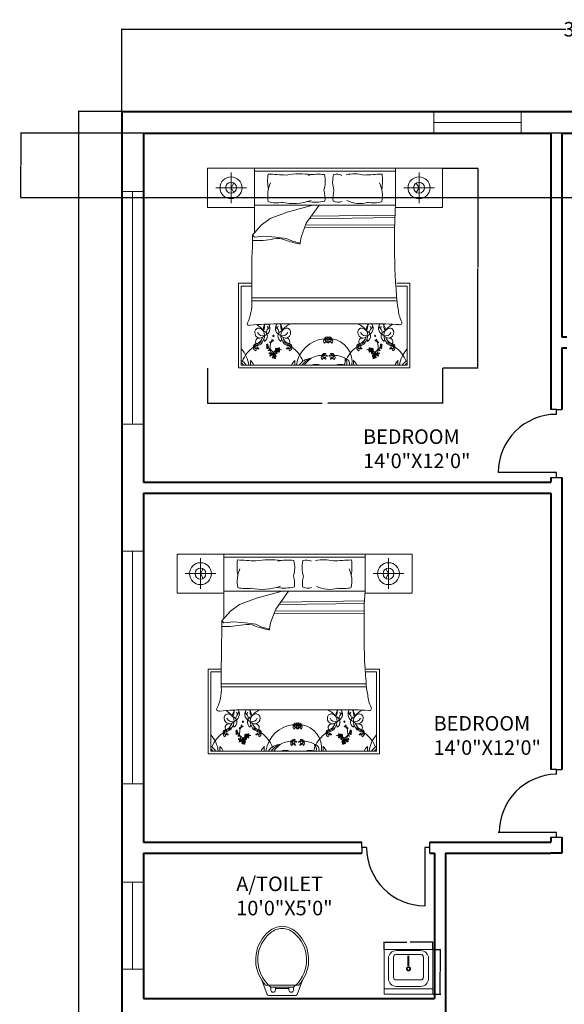
# Model space of a CAD drawing. Units: inches. Extents: x -19 to 419, y -828 to 43.
# Tile 8 of 9: x -19 to 205, y -364 to 43. Entities that reach past the tile are written whole.
import ezdxf

# ---------------------------------------------------------------- set-up
doc = ezdxf.new("R2010")
doc.units = ezdxf.units.IN
doc.header["$MEASUREMENT"] = 0
for name, color, linetype, lineweight in [('A-ANNO-DIMS', 2, 'Continuous', 18), ('A-AREA-IDEN', 7, 'Continuous', 25), ('A-DOOR', 3, 'Continuous', 25), ('A-FLOR-FIXT', 9, 'Continuous', 20), ('A-FURN', 8, 'Continuous', 18), ('A-GLAZ', 4, 'Continuous', 20), ('A-WALL', 7, 'Continuous', 40)]:
    doc.layers.add(name, color=color, linetype=linetype, lineweight=lineweight)
doc.styles.get("Standard").update_dxf_attribs({"font": 'arial.ttf'})
doc.dimstyles.get("Standard").update_dxf_attribs({"dimtxt": 0.18, "dimasz": 0.18, "dimexe": 0.18, "dimexo": 0.0625, "dimgap": 0.09, "dimtad": 0, "dimtih": 1, "dimtoh": 1, "dimdec": 0, "dimzin": 0, "dimdsep": 46, "dimlunit": 3, "dimtxsty": 'Standard', "dimcen": 0.09, "dimadec": 0, "dimazin": 0, "dimtfac": 1, "dimtdec": 0, "dimtofl": 0, "dimtmove": 0, "dimatfit": 3, "dimfxl": 1, "dimtolj": 1, "dimtzin": 0, "dimarcsym": 0})

# ---------------------------------------------------------------- blocks, each defined once
blk = doc.blocks.new('*D1')
at = {"layer": 'A-ANNO-DIMS', "color": 0, "lineweight": -2, "transparency": 16777216}
for p, q in [((22.74, 4.83), (22.74, 38.87)), ((22.92, 38.69), (205.85, 38.69)), ((409.56, 38.69), (226.63, 38.69)), ((409.74, 4.83), (409.74, 38.87))]:
    blk.add_line(p, q, dxfattribs=at)
at = {"layer": 'A-ANNO-DIMS', "color": 0, "transparency": 16777216}
for points in [[(22.92, 38.72), (22.92, 38.66), (22.74, 38.69)], [(409.56, 38.72), (409.56, 38.66), (409.74, 38.69)]]:
    blk.add_solid(points, dxfattribs=at)
at = {"layer": 'Defpoints', "color": 0, "transparency": 16777216}
for p in [(409.74, 38.69), (22.74, 4.77), (409.74, 4.77)]:
    blk.add_point(p, dxfattribs=at)
at = {"layer": 'A-ANNO-DIMS', "color": 0, "transparency": 16777216, "insert": (216.24, 38.69), "char_height": 6, "attachment_point": 5}
blk.add_mtext('\\A1;32\'-3"', dxfattribs=at)
blk = doc.blocks.new('*D2')
at = {"layer": 'A-ANNO-DIMS', "color": 0, "lineweight": -2, "transparency": 16777216}
for p, q in [((22.68, 4.77), (4.74, 4.77)), ((4.92, 4.59), (4.92, -387.33)), ((4.92, -785.55), (4.92, -393.64)), ((22.68, -785.73), (4.74, -785.73))]:
    blk.add_line(p, q, dxfattribs=at)
at = {"layer": 'A-ANNO-DIMS', "color": 0, "transparency": 16777216}
for points in [[(4.89, 4.59), (4.95, 4.59), (4.92, 4.77)], [(4.89, -785.55), (4.95, -785.55), (4.92, -785.73)]]:
    blk.add_solid(points, dxfattribs=at)
at = {"layer": 'Defpoints', "color": 0, "transparency": 16777216}
for p in [(22.74, 4.77), (4.92, -785.73), (22.74, -785.73)]:
    blk.add_point(p, dxfattribs=at)
at = {"layer": 'A-ANNO-DIMS', "color": 0, "transparency": 16777216, "insert": (4.92, -390.48), "char_height": 6, "attachment_point": 5}
blk.add_mtext('\\A1;65\'-11"', dxfattribs=at)
blk = doc.blocks.new('М14 600х655')
for p, q in [((-655, 600), (-655, 0)), ((-655, 600), (-655, 0)), ((-655, 0), (-655, 600)), ((0, 600), (-655, 600)), ((0, 0), (0, 600)), ((0, 525), (-655, 525)), ((-165, 494), (-490, 494)), ((-165, 408), (-490, 408)), ((-596, 388), (-596, 121)), ((-528, 370), (-528, 103)), ((-127, 103), (-127, 370)), ((-59, 121), (-59, 388)), ((-334, 87), (-334, 220)), ((-321, 87), (-321, 220)), ((-655, 0), (-655, 0)), ((-655, 0), (-655, 0)), ((-655, 0), (0, 0)), ((-655, 0), (0, 0)), ((-490, 65), (-165, 65)), ((-490, 15), (-165, 15))]:
    blk.add_line(p, q)
for radius in [27.6, 19.3]:
    blk.add_circle((-327, 259), radius)
for centre, radius, start, end in [((-490, 388), 106, 90, 180), ((-490, 370), 38.2, 90, 180), ((-165, 388), 106, 0, 90), ((-165, 370), 38.2, 0, 90), ((-490, 121), 106, 180, 270), ((-490, 103), 38.2, 180, 270), ((-165, 121), 106, 270, 0), ((-165, 103), 38.2, 270, 0)]:
    blk.add_arc(centre, radius, start, end)
blk = doc.blocks.new('WIN-36X9')
for p, q in [((36, 9), (0, 9)), ((0, 9), (0, 0)), ((36, 0), (36, 9)), ((0, 4.5), (36, 4.5)), ((0, 0), (36, 0))]:
    blk.add_line(p, q)
blk = doc.blocks.new('WIN-96X9')
for p, q in [((96, 9), (0, 9)), ((0, 9), (0, 0)), ((96, 0), (96, 9)), ((0, 4.5), (96, 4.5)), ((0, 0), (96, 0))]:
    blk.add_line(p, q)
blk = doc.blocks.new('DOOR-24-PARTITION')
for p, q in [((2, 2.25), (2, 26.25)), ((0, 4.5), (0, 0)), ((28, 2.25), (28, 4.5)), ((0, 2.25), (2, 2.25)), ((26, 2.25), (28, 2.25)), ((28, 2.25), (28, 0))]:
    blk.add_line(p, q)
blk.add_arc((2, 2.25), 24, 0, 90)
blk = doc.blocks.new('BED-DOUBLE-WITH-NIGHTSTANDS')
for p, q in [((0, 82.42), (96.91, 82.42)), ((19.38, 82.42), (19.38, 55.82)), ((9.69, 68.01), (9.69, 80.67)), ((77.53, 81.17), (19.38, 81.17)), ((87.22, 68.01), (87.22, 80.67)), ((16.02, 74.34), (3.36, 74.34)), ((80.89, 74.34), (93.55, 74.34)), ((19.38, 67.1), (77.53, 67.1)), ((32.84, 64.22), (43.41, 67.1)), ((46.01, 67.1), (40.69, 59.71)), ((22.05, 58.92), (25.78, 61.67)), ((25.78, 61.67), (32.84, 64.22)), ((77.23, 62.08), (42.04, 61.58)), ((77.27, 63.07), (42.77, 62.59)), ((18.51, 54.8), (22.05, 58.92)), ((40.69, 59.71), (38.54, 54.02)), ((77.19, 58.03), (40, 57.88)), ((77.18, 59.03), (40.38, 58.88)), ((19.3, 54.02), (18.51, 54.8)), ((23.23, 54.41), (19.3, 54.02)), ((28.13, 54.02), (23.23, 54.41)), ((32.45, 53.43), (28.13, 54.02)), ((35, 52.25), (32.45, 53.43)), ((38.54, 54.02), (38.14, 51.47)), ((38.14, 51.47), (35, 52.25)), ((12.79, 34.91), (18.27, 34.91)), ((12.79, 0), (12.79, 34.91)), ((18.27, 33.79), (13.91, 33.79)), ((13.91, 33.79), (13.91, 1.12)), ((82.32, 33.79), (78.05, 33.79)), ((78.07, 34.91), (83.44, 34.91)), ((82.32, 1.12), (82.32, 33.79)), ((83.44, 34.91), (83.44, 0)), ((77.97, 28.87), (18.27, 28.87)), ((78.06, 27.66), (18.27, 27.66)), ((68.13, 18.14), (28.78, 18.14)), ((23.46, 10.95), (23.25, 12.04)), ((30.24, 10.95), (30.45, 12.04)), ((66, 10.95), (65.78, 12.04)), ((72.77, 10.95), (72.98, 12.04)), ((13.91, 1.12), (82.32, 1.12)), ((83.44, 0), (12.79, 0))]:
    blk.add_line(p, q)
for points in [[(19.38, 66.26), (0, 66.26), (0, 82.42)], [(77.53, 82.42), (77.53, 66.26), (96.91, 66.26), (96.91, 82.42)], [(9.69, 74.34), (10.82, 76.3)], [(9.69, 74.34), (10.82, 72.38)], [(87.22, 74.34), (86.09, 76.3)], [(87.22, 74.34), (86.09, 72.38)]]:
    blk.add_lwpolyline(points)
for points in [[(24.95, 80, 0.074897), (25.07, 73.67, -0.472817)], [(48, 73.32, 0.14099), (48.19, 79.77, 0.235245)], [(52.14, 73.32, -0.14099), (51.95, 79.77, -0.235245)], [(71.96, 80, -0.074897), (71.84, 73.67, 0.472817)], [(18.31, 45.93, 0.001242), (18.27, 27.54, -0.127202), (16.32, 18.38)], [(77.94, 29.63, 0.056112), (78.64, 24.3, 0.095341), (80.01, 19.16)]]:
    blk.add_lwpolyline(points, format="xyb")
for centre, radius in [((9.69, 74.34), 4.52), ((87.22, 74.34), 4.52), ((9.69, 74.34), 2.26), ((87.22, 74.34), 2.26), ((27.45, 4.83), 0.247), ((29.06, 7.44), 0.247), ((67.17, 7.44), 0.247), ((68.79, 4.83), 0.247)]:
    blk.add_circle(centre, radius)
for centre, radius, start, end in [((78.36, 1002.26), 923.81, 266.68521, 267.14978), ((38.23, 44.93), 35.15, 82.2196, 99.497), ((45.65, 62.69), 17.27, 81.5249, 103.96), ((53.28, 75.17), 4.79, 63.3437, 106.1026), ((60.46, 63.04), 17.04, 76.3427, 101.1841), ((18.55, 1002.26), 923.81, 272.85022, 273.31479), ((37.29, 71.13), 12.49, 155.1316, 191.7583), ((36.58, 70.08), 11.87, 354.0129, 15.8293), ((63.56, 70.08), 11.87, 164.1707, 185.9871), ((59.62, 71.13), 12.49, 348.2417, 24.8684), ((35.24, 90.37), 22.53, 258.0397, 289.2615), ((62.9, 80.18), 12.34, 243.8761, 286.1746), ((28.41, 81.13), 12.99, 255.1039, 281.0369), ((44.36, 85.45), 17.09, 259.8617, 283.6238), ((53.92, 73.5), 5.14, 245.0183, 288.5407), ((68.5, 81.13), 12.99, 258.9631, 284.8961), ((251.26, 55.26), 174.13, 176.1, 180.9282), ((-70.34, 52.4), 88.89, 355.8294, 1.553), ((20.17, 89.12), 36.58, 267.4519, 281.3392), ((28.92, 45.53), 7.89, 66.2616, 101.3392), ((44.87, 88.09), 37.58, 250.1194, 259.3383), ((37.92, 51.39), 0.234, 268.8623, 19.7536), ((304.27, 48.93), 227.15, 179.1145, 184.8735), ((17.21, 18.44), 0.894, 183.98, 297.3412), ((27.63, -82.74), 100.88, 89.3433, 95.6887), ((21.11, 14.83), 1.64, 84.4856, 181.0538), ((16.84, 11.31), 7.33, 33.6671, 63.2997), ((20.61, 13.62), 2.91, 355.2933, 76.921), ((26.67, 15.68), 3.74, 145.785, 184.7304), ((19.53, 17.42), 4.02, 328.8218, 9.1554), ((24.5, 17.07), 1.17, 120.0293, 142.325), ((22.64, 16.38), 3.09, 289.2822, 29.1751), ((22.17, 15.82), 2.79, 7.436, 29.9149), ((24.01, 17.3), 1.45, 311.5653, 23.8354), ((24.5, 17.07), 1.17, 44.4517, 63.558), ((31.06, 16.38), 3.09, 150.8249, 250.7178), ((29.69, 17.3), 1.45, 156.1646, 228.4347), ((29.2, 17.07), 1.17, 113.229, 135.5483), ((31.53, 15.82), 2.79, 150.0851, 172.564), ((29.2, 17.07), 1.17, 37.675, 66.7144), ((27.03, 15.68), 3.74, 355.2696, 34.215), ((34.17, 17.42), 4.02, 169.7133, 211.1782), ((33.09, 13.62), 2.91, 103.079, 184.7067), ((36.86, 11.31), 7.33, 111.4941, 146.3329), ((32.59, 14.83), 1.64, 358.9462, 95.5144), ((63.64, 14.83), 1.64, 84.4856, 181.0538), ((59.37, 11.31), 7.33, 33.6671, 68.5059), ((63.14, 13.62), 2.91, 355.2933, 76.921), ((69.2, 15.68), 3.74, 145.785, 184.7304), ((62.06, 17.42), 4.02, 328.8218, 10.2867), ((67.03, 17.07), 1.17, 113.2856, 142.325), ((65.17, 16.38), 3.09, 289.2822, 29.1751), ((64.7, 15.82), 2.79, 7.436, 29.9149), ((67.03, 17.07), 1.17, 44.4517, 66.7144), ((66.54, 17.3), 1.45, 311.5653, 23.8354), ((71.1, -76.12), 94.3, 85.2402, 91.8035), ((73.6, 16.38), 3.09, 150.8249, 250.7178), ((72.23, 17.3), 1.45, 156.1646, 228.4347), ((71.73, 17.07), 1.17, 106.6343, 135.5483), ((74.06, 15.82), 2.79, 150.0851, 172.564), ((71.73, 17.07), 1.17, 37.675, 72.5814), ((69.57, 15.68), 3.74, 355.2696, 34.215), ((76.71, 17.42), 4.02, 169.249, 211.1782), ((75.63, 13.62), 2.91, 103.079, 184.7067), ((79.4, 11.31), 7.33, 113.6453, 146.3329), ((75.12, 14.83), 1.64, 358.9462, 95.5144), ((79.27, 18.67), 0.883, 246.5219, 33.8264), ((21.78, 14.6), 2.32, 174.9449, 262.8857), ((21.25, 10.87), 1.45, 80.264, 250.8688), ((22.69, 15.48), 2.25, 201.5819, 291.4221), ((18.36, 14.07), 4.58, 301.2614, 341.7045), ((21.38, 15.12), 2.82, 272.3591, 324.0401), ((18.32, 13.7), 5.2, 326.2883, 356.5076), ((22.26, 13.04), 2.41, 299.9085, 73.1337), ((26.67, 15.68), 3.74, 212.7011, 216.3445), ((23.79, 14.05), 0.601, 257.3041, 15.1471), ((26.29, 14.73), 1.99, 131.5653, 195.1471), ((27.13, 13.14), 0.187, 102.7051, 280.4384), ((27.11, 13.25), 0.304, 280.4384, 100.4136), ((27.41, 14.73), 1.99, 344.8529, 48.4347), ((31.44, 13.04), 2.41, 106.8663, 240.0915), ((29.91, 14.05), 0.601, 164.8529, 282.6959), ((27.03, 15.68), 3.74, 323.6555, 327.2989), ((32.32, 15.12), 2.82, 215.9599, 267.6409), ((31.01, 15.48), 2.25, 248.5779, 338.4181), ((35.38, 13.7), 5.2, 183.4924, 213.7117), ((35.34, 14.07), 4.58, 198.2955, 238.7386), ((31.92, 14.6), 2.32, 277.1143, 5.0551), ((32.45, 10.87), 1.45, 289.1312, 99.736), ((49.23, 11.74), 1.05, 63.0274, 163.8037), ((48.17, 14.19), 2.16, 271.4585, 315.3727), ((49.05, 10.21), 2, 45.5411, 114.3101), ((50.42, 10.21), 2, 65.6899, 134.4589), ((50.23, 11.74), 1.05, 16.1963, 116.9726), ((51.3, 14.19), 2.16, 224.6273, 268.5415), ((64.31, 14.6), 2.32, 174.9449, 262.8857), ((63.78, 10.87), 1.45, 80.264, 250.8688), ((65.22, 15.48), 2.25, 201.5819, 291.4221), ((60.9, 14.07), 4.58, 301.2614, 341.7045), ((63.91, 15.12), 2.82, 272.3591, 324.0401), ((60.85, 13.7), 5.2, 326.2883, 356.5076), ((64.8, 13.04), 2.41, 299.9085, 73.1337), ((69.2, 15.68), 3.74, 212.7011, 216.3445), ((66.32, 14.05), 0.601, 257.3041, 15.1471), ((68.82, 14.73), 1.99, 131.5653, 195.1471), ((69.13, 13.25), 0.304, 79.5864, 259.5616), ((69.11, 13.14), 0.187, 259.5616, 77.2949), ((69.95, 14.73), 1.99, 344.8529, 48.4347), ((73.97, 13.04), 2.41, 106.8663, 240.0915), ((72.45, 14.05), 0.601, 164.8529, 282.6959), ((69.57, 15.68), 3.74, 323.6555, 327.2989), ((74.86, 15.12), 2.82, 215.9599, 267.6409), ((73.54, 15.48), 2.25, 248.5779, 338.4181), ((77.91, 13.7), 5.2, 183.4924, 213.7117), ((77.87, 14.07), 4.58, 198.2955, 238.7386), ((74.45, 14.6), 2.32, 277.1143, 5.0551), ((74.99, 10.87), 1.45, 289.1312, 99.736), ((26.14, -1.83), 12.66, 124.3865, 158.5908), ((20.37, 8.31), 1.4, 167.7115, 249.0387), ((20.02, 8.86), 1.05, 92.9516, 193.728), ((17.87, 10.46), 2.16, 301.3827, 345.2969), ((20.62, 7.44), 2, 75.4653, 144.2343), ((17.08, 17.25), 8.85, 282.5173, 297.1824), ((18.96, 7.55), 1.06, 328.4633, 88.2869), ((21.1, 11.02), 3.2, 228.8402, 267.9352), ((19.91, 9.09), 1.04, 207.6827, 313.7762), ((20.95, 9.29), 0.891, 63.9755, 143.2681), ((20.53, 8.44), 0.137, 313.7762, 249.7183), ((20.9, 11.31), 1.82, 265.969, 344.3045), ((20.98, 8.06), 0.0763, 101.4834, 217.9409), ((20.99, 7.98), 0.157, 267.9352, 101.4834), ((22.85, 8.89), 1.93, 96.1662, 141.5825), ((24.62, 9.29), 0.412, 101.5637, 142.6358), ((24.28, 8.9), 0.247, 273.2768, 86.7232), ((24.61, 8.45), 0.407, 217.7621, 259.0403), ((24.57, 9.14), 0.236, 91.1081, 181.8675), ((25.05, 8.99), 0.749, 203.4276, 227.6104), ((24.82, 8.66), 0.51, 80.3487, 133.6538), ((24.73, 9.08), 0.404, 229.7889, 317.6792), ((24.29, 9.61), 0.593, 288.7263, 352.5032), ((24.27, 8.23), 0.574, 355.053, 68.3618), ((24.72, 8.13), 0.808, 83.0852, 105.7171), ((24.69, 9.58), 0.191, 345.2356, 144.9248), ((24.65, 8.2), 0.189, 232.4737, 355.053), ((19.12, 1.43), 9.2, 43.1541, 52.0459), ((24.87, 8.96), 0.213, 317.6792, 80.3487), ((26.06, 10.25), 0.509, 101.3256, 154.4621), ((25.33, 11.98), 1.53, 280.2588, 300.656), ((25.68, 13.2), 2.73, 268.3264, 277.1302), ((33.85, 8.26), 8.03, 163.5842, 183.8277), ((25, 11.97), 1.56, 308.2101, 316.3071), ((25.95, 10.95), 0.465, 278.3432, 4.2869), ((25.69, 11.36), 0.812, 300.656, 332.6341), ((26.3, 10.82), 0.197, 55.7657, 157.4417), ((33.85, 8.26), 8.03, 153.0032, 159.8941), ((26.61, 11), 0.197, 84.3784, 186.0543), ((26.43, 11.8), 0.812, 269.1859, 301.164), ((26.66, 11.38), 0.465, 237.5332, 323.4768), ((26.21, 12.7), 1.56, 285.5129, 293.6099), ((27.23, 10.95), 0.509, 87.3579, 140.4944), ((26.05, 12.41), 1.53, 301.164, 321.5612), ((24.81, 12.68), 2.73, 324.6898, 333.4936), ((29.4, 7.82), 0.412, 101.5637, 176.365), ((29.48, 8.11), 0.191, 345.2356, 144.9248), ((30.85, 8.89), 1.93, 38.4175, 83.8338), ((32.8, 11.31), 1.82, 195.6955, 274.031), ((32.75, 9.29), 0.891, 36.7319, 116.0245), ((32.71, 7.98), 0.157, 78.5166, 272.0648), ((33.08, 7.44), 2, 35.7657, 104.5347), ((36.62, 17.25), 8.85, 242.8176, 257.4827), ((32.6, 11.02), 3.2, 272.0648, 311.1598), ((32.72, 8.06), 0.0763, 322.0591, 78.5166), ((33.79, 9.09), 1.04, 226.2238, 332.3173), ((33.18, 8.49), 0.0825, 290.2667, 226.2271), ((34.74, 7.55), 1.06, 91.7131, 211.5367), ((33.69, 8.86), 1.05, 346.272, 87.0484), ((35.83, 10.46), 2.16, 194.7031, 238.6173), ((33.33, 8.31), 1.4, 290.9613, 12.2885), ((27.56, -1.83), 12.66, 21.4092, 55.6135), ((49.21, -0.58), 12.66, 94.4623, 172.255), ((49.26, 11.09), 1.4, 137.7873, 219.1145), ((47.67, 11.13), 1.06, 298.5391, 58.3627), ((50.87, 20.48), 8.85, 252.593, 267.2582), ((49.26, 11.99), 1.04, 177.7585, 283.852), ((51.25, 13.07), 3.2, 198.9159, 238.011), ((48.59, 20.48), 8.85, 272.7418, 287.407), ((49.47, 11.12), 0.137, 283.852, 219.9245), ((49.64, 10.49), 0.157, 238.011, 71.5592), ((49.66, 10.57), 0.0763, 71.5592, 188.0167), ((49.82, 10.49), 0.157, 108.4408, 301.989), ((49.8, 10.57), 0.0763, 351.9833, 108.4408), ((49.98, 11.17), 0.0825, 320.1909, 256.0209), ((48.21, 13.07), 3.2, 301.989, 341.0841), ((50.21, 11.99), 1.04, 256.148, 2.2415), ((51.79, 11.13), 1.06, 121.6373, 241.4609), ((50.2, 11.09), 1.4, 320.8855, 42.2127), ((49.85, 2.34), 9.79, 352.8636, 81.8197), ((68.68, -1.83), 12.66, 124.3865, 158.5908), ((62.55, 8.86), 1.05, 92.9516, 193.728), ((62.9, 8.31), 1.4, 167.7115, 249.0387), ((60.4, 10.46), 2.16, 301.3827, 345.2969), ((63.15, 7.44), 2, 75.4653, 144.2343), ((59.61, 17.25), 8.85, 282.5173, 297.1824), ((62.45, 9.09), 1.04, 207.6827, 313.7762), ((63.64, 11.02), 3.2, 228.8402, 267.9352), ((61.5, 7.55), 1.06, 328.4633, 88.2869), ((63.48, 9.29), 0.891, 63.9755, 143.2681), ((63.07, 8.44), 0.137, 313.7762, 249.7183), ((63.43, 11.31), 1.82, 265.969, 344.3045), ((63.51, 8.06), 0.0763, 101.4834, 217.9409), ((63.53, 7.98), 0.157, 267.9352, 101.4834), ((65.39, 8.89), 1.93, 96.1662, 141.5825), ((66.76, 8.11), 0.191, 35.0752, 194.7644), ((66.83, 7.82), 0.412, 3.635, 78.4363), ((70.18, 12.41), 1.53, 218.4388, 238.836), ((69, 10.95), 0.509, 39.5056, 92.6421), ((71.43, 12.68), 2.73, 206.5064, 215.3102), ((69.57, 11.38), 0.465, 216.5232, 302.4668), ((69.81, 11.8), 0.812, 238.836, 270.8141), ((70.02, 12.7), 1.56, 246.3901, 254.4871), ((62.39, 8.26), 8.03, 20.1059, 26.9968), ((69.62, 11), 0.197, 353.9457, 95.6216), ((69.93, 10.82), 0.197, 22.5583, 124.2343), ((70.28, 10.95), 0.465, 175.7131, 261.6568), ((70.54, 11.36), 0.812, 207.3659, 239.344), ((62.39, 8.26), 8.03, 356.1723, 16.4158), ((71.24, 11.97), 1.56, 223.6929, 231.7899), ((70.91, 11.98), 1.53, 239.344, 259.7412), ((70.55, 13.2), 2.73, 262.8698, 271.6736), ((70.18, 10.25), 0.509, 25.5379, 78.6744), ((77.11, 1.43), 9.2, 127.9541, 136.8459), ((71.37, 8.96), 0.213, 99.6513, 222.3208), ((71.51, 9.08), 0.404, 222.3208, 310.2111), ((71.42, 8.66), 0.51, 46.3462, 99.6513), ((71.54, 9.58), 0.191, 35.0752, 194.7644), ((71.94, 9.61), 0.593, 187.4968, 251.2737), ((71.96, 8.23), 0.574, 111.6382, 184.947), ((71.58, 8.2), 0.189, 184.947, 307.5263), ((71.51, 8.13), 0.808, 74.2829, 96.9148), ((71.67, 9.14), 0.236, 358.1325, 88.8919), ((71.18, 8.99), 0.749, 312.3896, 336.5724), ((71.61, 9.29), 0.412, 37.3642, 78.4363), ((71.62, 8.45), 0.407, 280.9597, 322.2379), ((71.96, 8.9), 0.247, 93.2768, 266.7232), ((75.34, 11.31), 1.82, 195.6955, 274.031), ((73.38, 8.89), 1.93, 38.4175, 83.8338), ((75.29, 9.29), 0.891, 36.7319, 116.0245), ((75.24, 7.98), 0.157, 78.5166, 272.0648), ((75.61, 7.44), 2, 35.7657, 104.5347), ((79.16, 17.25), 8.85, 242.8176, 257.4827), ((75.13, 11.02), 3.2, 272.0648, 311.1598), ((75.26, 8.06), 0.0763, 322.0591, 78.5166), ((76.32, 9.09), 1.04, 226.2238, 332.3173), ((75.71, 8.49), 0.0825, 290.2667, 226.2271), ((77.27, 7.55), 1.06, 91.7131, 211.5367), ((78.36, 10.46), 2.16, 194.7031, 238.6173), ((76.22, 8.86), 1.05, 346.272, 87.0484), ((75.87, 8.31), 1.4, 290.9613, 12.2885), ((70.09, -1.83), 12.66, 21.4092, 55.6135), ((4.49, -0.58), 12.66, 7.745, 41.8856), ((25.48, 6.99), 0.509, 101.3256, 154.4621), ((24.75, 8.72), 1.53, 280.2588, 300.656), ((25.1, 9.94), 2.73, 268.3264, 277.1302), ((24.42, 8.71), 1.56, 308.2101, 316.3071), ((25.65, 6.1), 0.276, 146.8636, 236.9021), ((29.54, 12.17), 7.21, 235.1882, 238.8844), ((26.13, 6.5), 0.746, 199.4799, 267.6828), ((25.37, 7.69), 0.465, 278.3432, 4.2869), ((26.04, 6.21), 0.643, 212.8155, 277.3992), ((25.12, 8.1), 0.812, 300.656, 332.6341), ((25.73, 7.56), 0.197, 55.7657, 157.4417), ((25.67, 5.78), 0.746, 266.9701, 338.2913), ((21.74, 11.11), 7.21, 302.6784, 306.3746), ((25.86, 5.19), 0.276, 214.3538, 304.3923), ((25.96, 6.24), 0.285, 238.8844, 314.2646), ((29.85, 8.06), 4.02, 184.756, 209.2041), ((35.64, 16.62), 13.24, 222.2412, 232.1744), ((25.9, 5.6), 0.643, 280.3057, 17.1958), ((25.84, 5.53), 0.285, 306.3746, 21.7548), ((26.31, 5.72), 0.215, 19.3605, 201.7548), ((26.31, 5.88), 0.215, 311.8703, 134.2646), ((30.36, 3.92), 4.3, 153.7819, 158.2913), ((26.93, 6.85), 1.12, 247.2305, 319.0635), ((26.56, 6.48), 0.662, 264.4544, 310.6188), ((29.85, 8.06), 4.02, 214.0033, 222.4917), ((27.05, 6.21), 0.684, 218.3208, 298.8162), ((30.26, 2.71), 4.83, 120.544, 139.818), ((26.93, 4.37), 0.245, 148.0499, 225.6268), ((27.38, 4.09), 0.778, 104.7558, 148.0499), ((26.95, 4.65), 0.487, 247.4086, 351.4386), ((27.18, 5.18), 0.337, 126.1046, 271.4281), ((27.14, 5.27), 0.242, 353.7526, 131.7054), ((27.51, 5.37), 0.796, 70.0041, 130.6188), ((27.08, 4.63), 0.163, 262.906, 7.132), ((26.91, 4.98), 0.34, 0.0645, 61.1507), ((26.99, 5.27), 0.388, 311.8413, 355.7877), ((27, 6.34), 0.817, 297.7043, 344.3516), ((27.79, 5.22), 0.412, 101.5637, 176.365), ((27.78, 4.38), 0.407, 151.2196, 259.0403), ((27.74, 5.07), 0.236, 91.1081, 181.8675), ((28.22, 4.92), 0.749, 203.4276, 227.6104), ((27.99, 4.59), 0.51, 80.3487, 133.6538), ((27.9, 5.02), 0.404, 229.7889, 317.6792), ((27.46, 5.54), 0.593, 288.7263, 352.5032), ((27.44, 4.16), 0.574, 355.053, 68.3618), ((27.89, 4.06), 0.808, 83.0852, 105.7171), ((27.86, 5.51), 0.191, 345.2356, 144.9248), ((27.82, 4.13), 0.189, 232.4737, 355.053), ((27.17, 7.8), 1.12, 304.5369, 16.3699), ((27.77, 7.55), 0.684, 272.8499, 356.1226), ((27.29, 7.29), 0.662, 321.7607, 7.9252), ((27.43, 6.33), 0.662, 8.7227, 54.8872), ((27.47, 5.81), 1.12, 0.278, 72.111), ((28.74, 7.49), 0.796, 127.3105, 187.9252), ((27.97, 6.22), 0.684, 20.5253, 88.5375), ((28.04, 4.89), 0.213, 317.6792, 80.3487), ((28.87, 6.56), 0.796, 188.7227, 249.3375), ((27.64, 7.58), 0.817, 355.0106, 41.658), ((28.54, 6.97), 0.245, 148.0499, 225.6268), ((30.26, 2.71), 4.83, 113.0501, 113.8477), ((29, 6.69), 0.778, 104.7558, 148.0499), ((28.56, 7.25), 0.487, 247.4086, 351.4386), ((28.79, 7.78), 0.337, 126.1046, 271.4281), ((28.75, 7.87), 0.242, 353.7526, 131.7054), ((27.85, 6.16), 0.817, 334.9899, 21.6373), ((28.7, 7.23), 0.163, 262.906, 7.132), ((28.53, 7.58), 0.34, 0.0645, 61.1507), ((28.61, 7.87), 0.388, 311.8413, 355.7877), ((29.4, 6.98), 0.407, 151.2196, 259.0403), ((29.35, 7.67), 0.236, 91.1081, 181.8675), ((29.84, 7.52), 0.749, 203.4276, 227.6104), ((29.6, 7.2), 0.51, 80.3487, 133.6538), ((29.51, 7.62), 0.404, 229.7889, 317.6792), ((29.07, 8.14), 0.593, 288.7263, 352.5032), ((29.05, 6.76), 0.574, 355.053, 68.3618), ((29.5, 6.67), 0.808, 83.0852, 105.7171), ((29.44, 6.73), 0.189, 232.4737, 355.053), ((29.65, 7.49), 0.213, 317.6792, 80.3487), ((30.26, 2.71), 4.83, 87.1071, 94.7585), ((48.24, -7.36), 12.66, 94.4623, 117.4146), ((48.29, 4.31), 1.4, 137.7873, 219.1145), ((46.7, 4.36), 1.06, 298.5391, 58.3627), ((48.26, 4.96), 1.05, 63.0274, 163.8037), ((47.2, 7.42), 2.16, 271.4585, 315.3727), ((48.08, 3.43), 2, 45.5411, 114.3101), ((50.28, 6.29), 3.2, 198.9159, 238.011), ((49.9, 13.7), 8.85, 252.593, 267.2582), ((48.29, 5.22), 1.04, 177.7585, 283.852), ((48.5, 4.34), 0.137, 283.852, 219.9245), ((51.39, 3.43), 2, 65.6899, 134.4589), ((49.56, 13.7), 8.85, 272.7418, 287.407), ((51.2, 4.96), 1.05, 16.1963, 116.9726), ((52.26, 7.42), 2.16, 224.6273, 268.5415), ((50.95, 4.4), 0.0825, 320.1909, 256.0209), ((49.18, 6.29), 3.2, 301.989, 341.0841), ((51.17, 5.22), 1.04, 256.148, 2.2415), ((52.76, 4.36), 1.06, 121.6373, 241.4609), ((51.17, 4.31), 1.4, 320.8855, 42.2127), ((51.22, -7.36), 12.66, 62.5854, 85.5377), ((65.97, 2.71), 4.83, 85.2415, 92.8929), ((66.58, 7.49), 0.213, 99.6513, 222.3208), ((66.72, 7.62), 0.404, 222.3208, 310.2111), ((66.63, 7.2), 0.51, 46.3462, 99.6513), ((67.16, 8.14), 0.593, 187.4968, 251.2737), ((67.18, 6.76), 0.574, 111.6382, 184.947), ((66.8, 6.73), 0.189, 184.947, 307.5263), ((66.73, 6.67), 0.808, 74.2829, 96.9148), ((66.88, 7.67), 0.236, 358.1325, 88.8919), ((66.39, 7.52), 0.749, 312.3896, 336.5724), ((66.83, 6.98), 0.407, 280.9597, 28.7804), ((67.67, 7.25), 0.487, 188.5614, 292.5914), ((67.48, 7.87), 0.242, 48.2946, 186.2474), ((67.63, 7.87), 0.388, 184.2123, 228.1587), ((67.71, 7.58), 0.34, 118.8493, 179.9355), ((67.54, 7.23), 0.163, 172.868, 277.094), ((67.44, 7.78), 0.337, 268.5719, 53.8954), ((67.24, 6.69), 0.778, 31.9501, 75.2442), ((68.38, 6.16), 0.817, 158.3627, 205.0101), ((68.26, 6.22), 0.684, 91.4625, 159.4747), ((68.77, 5.81), 1.12, 107.889, 179.722), ((67.36, 6.56), 0.796, 290.6625, 351.2773), ((68.59, 7.58), 0.817, 138.342, 184.9894), ((68.46, 7.55), 0.684, 183.8774, 267.1501), ((65.97, 2.71), 4.83, 66.1523, 66.9499), ((67.69, 6.97), 0.245, 314.3732, 31.9501), ((69.06, 7.8), 1.12, 163.6301, 235.4631), ((67.5, 7.49), 0.796, 352.0748, 52.6895), ((68.2, 4.89), 0.213, 99.6513, 222.3208), ((68.34, 5.02), 0.404, 222.3208, 310.2111), ((68.8, 6.33), 0.662, 125.1128, 171.2773), ((68.25, 4.59), 0.51, 46.3462, 99.6513), ((68.37, 5.51), 0.191, 35.0752, 194.7644), ((68.77, 5.54), 0.593, 187.4968, 251.2737), ((68.79, 4.16), 0.574, 111.6382, 184.947), ((68.41, 4.13), 0.189, 184.947, 307.5263), ((68.34, 4.06), 0.808, 74.2829, 96.9148), ((68.94, 7.29), 0.662, 172.0748, 218.2393), ((65.97, 2.71), 4.83, 40.182, 59.456), ((68.72, 5.37), 0.796, 49.3812, 109.9959), ((69.3, 6.85), 1.12, 220.9365, 292.7695), ((69.24, 6.34), 0.817, 195.6484, 242.2957), ((68.5, 5.07), 0.236, 358.1325, 88.8919), ((68.01, 4.92), 0.749, 312.3896, 336.5724), ((68.44, 5.22), 0.412, 3.635, 78.4363), ((68.45, 4.38), 0.407, 280.9597, 28.7804), ((60.59, 16.62), 13.24, 307.8256, 317.7588), ((69.29, 4.65), 0.487, 188.5614, 292.5914), ((69.1, 5.27), 0.242, 48.2946, 186.2474), ((69.24, 5.27), 0.388, 184.2123, 228.1587), ((69.19, 6.21), 0.684, 241.1838, 321.6792), ((69.32, 4.98), 0.34, 118.8493, 179.9355), ((69.15, 4.63), 0.163, 172.868, 277.094), ((69.06, 5.18), 0.337, 268.5719, 53.8954), ((68.85, 4.09), 0.778, 31.9501, 75.2442), ((69.67, 6.48), 0.662, 229.3812, 275.5456), ((66.39, 8.06), 4.02, 317.5083, 325.9967), ((69.3, 4.37), 0.245, 314.3732, 31.9501), ((70.34, 5.6), 0.643, 162.8042, 259.6943), ((69.92, 5.88), 0.215, 45.7354, 228.1297), ((69.93, 5.72), 0.215, 338.2452, 160.6395), ((65.88, 3.92), 4.3, 21.7087, 26.2181), ((70.57, 5.78), 0.746, 201.7087, 273.0299), ((66.39, 8.06), 4.02, 330.7959, 355.244), ((70.27, 6.24), 0.285, 225.7354, 301.1156), ((70.19, 6.21), 0.643, 262.6008, 327.1845), ((70.39, 5.53), 0.285, 158.2452, 233.6254), ((70.11, 6.5), 0.746, 272.3172, 340.5201), ((74.5, 11.11), 7.21, 233.6254, 237.3216), ((70.38, 5.19), 0.276, 235.6077, 325.6462), ((70.51, 7.56), 0.197, 22.5583, 124.2343), ((70.86, 7.69), 0.465, 175.7131, 261.6568), ((71.12, 8.1), 0.812, 207.3659, 239.344), ((66.7, 12.17), 7.21, 301.1156, 304.8118), ((71.82, 8.71), 1.56, 223.6929, 231.7899), ((71.48, 8.72), 1.53, 239.344, 259.7412), ((70.58, 6.1), 0.276, 303.0979, 33.1364), ((71.13, 9.94), 2.73, 262.8698, 271.6736), ((70.75, 6.99), 0.509, 25.5379, 78.6744), ((91.74, -0.58), 12.66, 138.1144, 172.255), ((10.84, -2.28), 6.17, 33.4617, 60.1116), ((8.62, -3.43), 7.68, 36.3036, 46.4814), ((14.3, -0.85), 5.15, 22.5547, 48.9546), ((0.2, 1.91), 17.51, 357.4081, 3.6519), ((39.41, -0.85), 5.15, 131.0454, 157.4453), ((53.5, 1.91), 17.51, 176.3481, 182.5919), ((42.86, -2.28), 6.17, 91.272, 146.5383), ((45.08, -3.43), 7.68, 107.8504, 143.6964), ((49.12, -5.59), 11.43, 124.0123, 144.053), ((44.7, -5.53), 6.96, 73.5431, 107.0202), ((47.46, -9.12), 10.29, 94.3787, 95.6357), ((52.88, -16.17), 18.39, 109.7217, 109.9028), ((48.67, 3.71), 0.157, 238.011, 71.5592), ((48.7, 3.79), 0.0763, 71.5592, 188.0167), ((50.79, 3.71), 0.157, 108.4408, 301.989), ((50.77, 3.79), 0.0763, 351.9833, 108.4408), ((54.76, -5.53), 6.96, 72.9798, 106.4569), ((52.01, -9.12), 10.29, 84.3643, 85.6213), ((46.59, -16.17), 18.39, 70.0972, 70.2783), ((51.11, 3.23), 5.67, 338.117, 6.6195), ((56.31, 1.66), 2.27, 346.3898, 79.0739), ((54.6, 1.97), 2.87, 342.8609, 41.9049), ((42.73, 1.91), 17.51, 357.4081, 3.6519), ((56.83, -0.85), 5.15, 22.5547, 48.9546), ((81.94, -0.85), 5.15, 131.0454, 157.4453), ((96.03, 1.91), 17.51, 176.3481, 182.5919), ((85.39, -2.28), 6.17, 119.8884, 146.5383), ((87.61, -3.43), 7.68, 133.5186, 143.6964)]:
    blk.add_arc(centre, radius, start, end)
blk = doc.blocks.new('WC-FLOOR-MOUNT')
for p, q in [((4.1, 4.33), (5.3, 4.33)), ((5.3, 4.33), (10.92, 4.33)), ((16.55, 4.33), (10.92, 4.33)), ((16.55, 4.33), (17.75, 4.33))]:
    blk.add_line(p, q)
for points in [[(2.55, 6.29, -0.383919), (5.55, 26.53, -0.163732), (10.92, 28.59, -0.359733)], [(19.29, 6.29, 0.383919), (16.3, 26.53, 0.163732), (10.92, 28.59, 0.359733)], [(4.72, 4.91, -0.431639), (6.09, 25.87, -0.162618), (10.92, 27.73, -0.470877)], [(16.55, 4.33, 0.448546), (15.75, 25.87, 0.162618), (10.92, 27.73, 0.470877)], [(4.1, 4.33, -0.040937), (2.55, 6.29, -0.163732)], [(10.92, 0), (5.46, 0, -0.31031), (4.79, 0.46), (2.55, 6.29, -0.209071)], [(5.3, 4.33, -0.014165), (4.72, 4.91, -0.162618)], [(6.28, 3.47, -0.022712), (5.3, 4.33, -0.162618)], [(10.92, 0), (16.38, 0, 0.31031), (17.05, 0.46), (19.29, 6.29, 0.209071)], [(15.56, 3.47, 0.022712), (16.55, 4.33, 0.162618)], [(17.75, 4.33, 0.040937), (19.29, 6.29, 0.163732)], [(10.92, 3.47), (6.28, 3.47, -0.022712)], [(6.28, 3.47), (6.28, 2.27, 1), (8.11, 2.27), (8.11, 2.89)], [(10.92, 3.47), (15.56, 3.47, 0.476108)], [(15.56, 3.47), (15.56, 2.27, -1), (13.74, 2.27), (13.74, 2.89)]]:
    blk.add_lwpolyline(points, format="xyb")
for points in [[(8.11, 2.89), (8.11, 3.47)], [(13.74, 2.89), (8.11, 2.89)], [(13.74, 2.89), (13.74, 3.47)]]:
    blk.add_lwpolyline(points)
blk = doc.blocks.new('*D26')
at = {"layer": 'A-ANNO-DIMS', "color": 0, "lineweight": -2, "transparency": 16777216}
for p, q in [((58.13, -101.13), (58.13, -115.79)), ((155.04, -101.13), (155.04, -115.79)), ((58.31, -115.61), (105.37, -115.61)), ((154.86, -115.61), (107.79, -115.61))]:
    blk.add_line(p, q, dxfattribs=at)
at = {"layer": 'A-ANNO-DIMS', "color": 0, "transparency": 16777216}
for points in [[(58.31, -115.58), (58.31, -115.64), (58.13, -115.61)], [(154.86, -115.58), (154.86, -115.64), (155.04, -115.61)]]:
    blk.add_solid(points, dxfattribs=at)
at = {"layer": 'Defpoints', "color": 0, "transparency": 16777216}
for p in [(58.13, -101.07), (155.04, -101.07), (155.04, -115.61)]:
    blk.add_point(p, dxfattribs=at)
at = {"layer": 'A-ANNO-DIMS', "color": 0, "transparency": 16777216, "insert": (106.58, -115.61), "char_height": 0.18, "attachment_point": 5}
blk.add_mtext('\\A1;BED SET 8\'-1" TYP.', dxfattribs=at)
blk = doc.blocks.new('*D27')
at = {"layer": 'A-ANNO-DIMS', "color": 0, "lineweight": -2, "transparency": 16777216}
for p, q in [((155.1, -18.66), (169.75, -18.66)), ((169.57, -18.84), (169.57, -59.68)), ((169.57, -100.89), (169.57, -60.05)), ((155.1, -101.07), (169.75, -101.07))]:
    blk.add_line(p, q, dxfattribs=at)
at = {"layer": 'A-ANNO-DIMS', "color": 0, "transparency": 16777216}
for points in [[(169.54, -18.84), (169.6, -18.84), (169.57, -18.66)], [(169.54, -100.89), (169.6, -100.89), (169.57, -101.07)]]:
    blk.add_solid(points, dxfattribs=at)
at = {"layer": 'Defpoints', "color": 0, "transparency": 16777216}
for p in [(155.04, -18.66), (169.57, -18.66), (155.04, -101.07)]:
    blk.add_point(p, dxfattribs=at)
at = {"layer": 'A-ANNO-DIMS', "color": 0, "transparency": 16777216, "insert": (169.57, -59.86), "char_height": 0.18, "attachment_point": 5}
blk.add_mtext('\\A1;6\'-10 1/2" TYP.', dxfattribs=at)
blk = doc.blocks.new('*D32')
at = {"layer": 'A-ANNO-DIMS', "color": 0, "lineweight": -2, "transparency": 16777216}
for p, q in [((130.9, -340.98), (130.9, -337.83)), ((131.08, -338.01), (140.25, -338.01)), ((150.9, -338.01), (141.73, -338.01)), ((151.08, -340.98), (151.08, -337.83))]:
    blk.add_line(p, q, dxfattribs=at)
at = {"layer": 'A-ANNO-DIMS', "color": 0, "transparency": 16777216}
for points in [[(131.08, -337.98), (131.08, -338.04), (130.9, -338.01)], [(150.9, -337.98), (150.9, -338.04), (151.08, -338.01)]]:
    blk.add_solid(points, dxfattribs=at)
at = {"layer": 'Defpoints', "color": 0, "transparency": 16777216}
for p in [(130.9, -341.04), (151.08, -338.01), (151.08, -341.04)]:
    blk.add_point(p, dxfattribs=at)
at = {"layer": 'A-ANNO-DIMS', "color": 0, "transparency": 16777216, "insert": (140.99, -338.01), "char_height": 0.18, "attachment_point": 5}
blk.add_mtext('\\A1;BASIN 1\'-8"', dxfattribs=at)
blk = doc.blocks.new('*D33')
at = {"layer": 'A-ANNO-DIMS', "color": 0, "lineweight": -2, "transparency": 16777216}
for p, q in [((151.15, -341.04), (154.29, -341.04)), ((154.11, -341.22), (154.11, -350.1)), ((154.11, -359.35), (154.11, -350.47)), ((151.15, -359.53), (154.29, -359.53))]:
    blk.add_line(p, q, dxfattribs=at)
at = {"layer": 'A-ANNO-DIMS', "color": 0, "transparency": 16777216}
for points in [[(154.08, -341.22), (154.14, -341.22), (154.11, -341.04)], [(154.08, -359.35), (154.14, -359.35), (154.11, -359.53)]]:
    blk.add_solid(points, dxfattribs=at)
at = {"layer": 'Defpoints', "color": 0, "transparency": 16777216}
for p in [(151.08, -341.04), (151.08, -359.53), (154.11, -359.53)]:
    blk.add_point(p, dxfattribs=at)
at = {"layer": 'A-ANNO-DIMS', "color": 0, "transparency": 16777216, "insert": (154.11, -350.29), "char_height": 0.18, "attachment_point": 5}
blk.add_mtext('\\A1;1\'-6 1/2"', dxfattribs=at)
blk = doc.blocks.new('*D47')
at = {"layer": 'A-ANNO-DIMS', "color": 0, "lineweight": -2, "transparency": 16777216}
for p, q in [((372.05, -4.23), (-19.04, -4.23)), ((-18.86, -4.41), (-18.86, -17.36)), ((-18.86, -30.67), (-18.86, -17.72)), ((372.05, -30.85), (-19.04, -30.85))]:
    blk.add_line(p, q, dxfattribs=at)
at = {"layer": 'A-ANNO-DIMS', "color": 0, "transparency": 16777216}
for points in [[(-18.89, -4.41), (-18.83, -4.41), (-18.86, -4.23)], [(-18.89, -30.67), (-18.83, -30.67), (-18.86, -30.85)]]:
    blk.add_solid(points, dxfattribs=at)
at = {"layer": 'Defpoints', "color": 0, "transparency": 16777216}
for p in [(-18.86, -4.23), (372.11, -4.23), (372.11, -30.85)]:
    blk.add_point(p, dxfattribs=at)
at = {"layer": 'A-ANNO-DIMS', "color": 0, "transparency": 16777216, "insert": (-18.86, -17.54), "char_height": 0.18, "attachment_point": 5}
blk.add_mtext('\\A1;2\'-2 1/2"', dxfattribs=at)

msp = doc.modelspace()

# ---------------------------------------------------------------- linework, layer by layer
at = {"layer": 'A-DOOR'}
for p, q in [((201.99, -266.73), (199.74, -266.73)), ((201.99, -268.73), (201.99, -266.73)), ((201.99, -266.73), (204.24, -266.73)), ((201.99, -292.73), (177.99, -292.73)), ((199.74, -294.73), (204.24, -294.73)), ((201.99, -294.73), (201.99, -292.73))]:
    msp.add_line(p, q, dxfattribs=at)
msp.add_arc((202.41, -292.73), 24, 90.9966, 180, dxfattribs=at)
at = {"layer": 'A-WALL'}
for p, q in [((22.74, 4.77), (22.74, -785.73)), ((22.74, 4.77), (409.74, 4.77)), ((31.74, -4.23), (199.74, -4.23)), ((31.74, -4.23), (31.74, -148.23)), ((199.74, -4.23), (199.74, -118.23)), ((204.24, -4.23), (204.24, -88.23)), ((204.24, -4.23), (276.24, -4.23)), ((204.24, -88.23), (206.24, -88.23)), ((204.24, -92.73), (206.24, -92.73)), ((204.24, -92.73), (204.24, -118.23)), ((199.74, -146.23), (199.74, -148.23)), ((204.24, -146.23), (204.24, -266.73)), ((31.74, -148.23), (199.74, -148.23)), ((31.74, -152.73), (199.74, -152.73)), ((31.74, -152.73), (31.74, -296.73)), ((199.74, -152.73), (199.74, -266.73)), ((199.74, -294.73), (199.74, -296.73)), ((204.24, -294.73), (204.24, -301.23)), ((31.74, -296.73), (121.74, -296.73)), ((149.74, -296.73), (199.74, -296.73)), ((31.74, -301.23), (121.74, -301.23)), ((31.74, -301.23), (31.74, -361.23)), ((149.74, -301.23), (151.74, -301.23)), ((151.74, -301.23), (151.74, -361.23)), ((156.24, -301.23), (156.24, -430.23)), ((156.24, -301.23), (199.74, -301.23)), ((204.24, -301.23), (199.74, -301.23)), ((31.74, -361.23), (151.74, -361.23))]:
    msp.add_line(p, q, dxfattribs=at)

# ---------------------------------------------------------------- block references
at = {"layer": 'A-DOOR'}
for p, rotation in [((204.24, -146.23), 90.00000000000011), ((149.74, -296.73), 180)]:
    msp.add_blockref('DOOR-24-PARTITION', p, dxfattribs=dict(at, rotation=rotation))
at = {"layer": 'A-FLOR-FIXT'}
msp.add_blockref('WC-FLOOR-MOUNT', (77.97, -360.05), dxfattribs=at)
at = {"layer": 'A-FLOR-FIXT', "xscale": -0.0308175584053277, "yscale": 0.0308175584053277, "zscale": 0.0308175584053277, "rotation": 180}
msp.add_blockref('М14 600х655', (151.08, -341.04), dxfattribs=at)
at = {"layer": 'A-FURN'}
for p in [(58.13, -101.07), (45.53, -260.29)]:
    msp.add_blockref('BED-DOUBLE-WITH-NIGHTSTANDS', p, dxfattribs=at)
at = {"layer": 'A-GLAZ'}
msp.add_blockref('WIN-36X9', (151.47, -4.23), dxfattribs=at)
for name, p, rotation in [('WIN-96X9', (22.74, -28.23), 270.0000000000002), ('WIN-96X9', (22.74, -176.73), 270.0000000000002), ('WIN-36X9', (22.74, -313.23), 269.9999999999999)]:
    msp.add_blockref(name, p, dxfattribs=dict(at, rotation=rotation))

# ---------------------------------------------------------------- texts
at = {"layer": 'A-AREA-IDEN', "char_height": 6, "attachment_point": 1}
for s, insert in [('BEDROOM\\P14\'0"X12\'0"', (122.27, -126.42)), ('BEDROOM\\P14\'0"X12\'0"', (151.35, -244.73)), ('A/TOILET\\P10\'0"X5\'0"', (69.98, -310.95))]:
    msp.add_mtext(s, dxfattribs=dict(at, insert=insert))

# ---------------------------------------------------------------- dimensions: what is measured, and where the dimension line sits
at = {"layer": 'A-ANNO-DIMS'}
dim = msp.add_linear_dim(base=(409.74, 38.69), p1=(22.74, 4.77), p2=(409.74, 4.77), dimstyle='Standard', override={"dimtxt": 6, "dimclrd": 0, "dimclre": 0, "dimclrt": 0}, dxfattribs=at)
dim.commit()
dim.dimension.update_dxf_attribs({"geometry": '*D1', "text_midpoint": (216.24, 38.69)})
for base, p1, p2, angle, override, picture, middle in [((4.917623, -785.73343372), (22.73889525, 4.76656628), (22.73889525, -785.73343372), 90, {"dimtxt": 6, "dimclrd": 0, "dimclre": 0, "dimclrt": 0}, '*D2', (4.917623, -390.48343372)), ((-18.86, -4.23), (372.11, -30.85), (372.11, -4.23), 90, {"dimdec": 1, "dimlfac": 1, "dimrnd": 0, "dimzin": 1, "dimdsep": 46, "dimlunit": 4, "dimfrac": 2}, '*D47', (-18.86, -17.54)), ((154.11, -359.53), (151.08, -341.04), (151.08, -359.53), 270, {"dimdec": 1, "dimlfac": 1, "dimrnd": 0, "dimzin": 1, "dimdsep": 46, "dimlunit": 4, "dimfrac": 2}, '*D33', (154.11, -350.29))]:
    dim = msp.add_linear_dim(base=base, p1=p1, p2=p2, angle=angle, dimstyle='Standard', override=override, dxfattribs=at)
    dim.commit()
    dim.dimension.update_dxf_attribs({"geometry": picture, "text_midpoint": middle})
dim = msp.add_linear_dim(base=(169.57, -18.66), p1=(155.04, -101.07), p2=(155.04, -18.66), angle=90, text='<> TYP.', dimstyle='Standard', override={"dimdec": 1, "dimlfac": 1, "dimrnd": 0, "dimzin": 1, "dimdsep": 46, "dimlunit": 4, "dimfrac": 2}, dxfattribs=at)
dim.commit()
dim.dimension.update_dxf_attribs({"geometry": '*D27', "text_midpoint": (169.57, -59.86)})
for base, p1, p2, text, picture, middle in [((155.04, -115.61), (58.13, -101.07), (155.04, -101.07), 'BED SET <> TYP.', '*D26', (106.58, -115.61)), ((151.08, -338.01), (130.9, -341.04), (151.08, -341.04), 'BASIN <>', '*D32', (140.99, -338.01))]:
    dim = msp.add_linear_dim(base=base, p1=p1, p2=p2, text=text, dimstyle='Standard', override={"dimdec": 1, "dimlfac": 1, "dimrnd": 0, "dimzin": 1, "dimdsep": 46, "dimlunit": 4, "dimfrac": 2}, dxfattribs=at)
    dim.commit()
    dim.dimension.update_dxf_attribs({"geometry": picture, "text_midpoint": middle})

doc.saveas('drawing.dxf')
